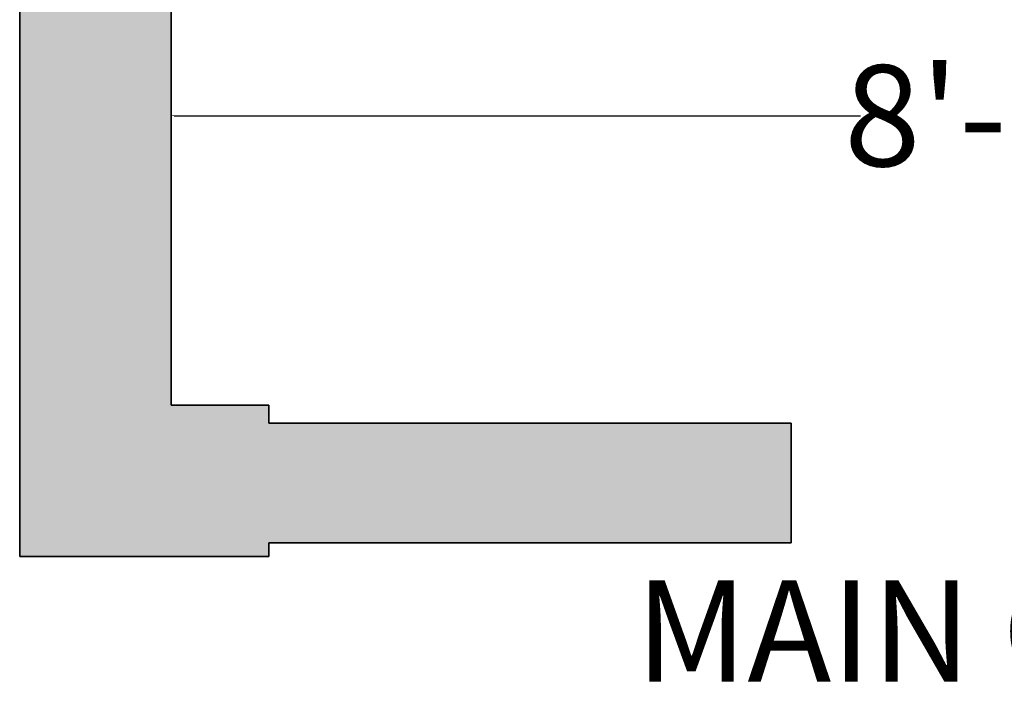
# Model space of a CAD drawing. Units: inches. Extents: x -5 to 482, y -460 to 66.
# Tile 1 of 31: x 33 to 91, y -429 to -390. Entities that reach past the tile are written whole.
import ezdxf

# ---------------------------------------------------------------- set-up
doc = ezdxf.new("R2010")
doc.units = ezdxf.units.IN
doc.header["$MEASUREMENT"] = 0
for name, color, linetype, lineweight in [('A-ANNO-DIMS', 2, 'Continuous', 18), ('A-ANNO-TEXT', 7, 'Continuous', 18), ('A-WALL', 7, 'Continuous', 35), ('A-WALL-PATT', 152, 'Continuous', 13)]:
    doc.layers.add(name, color=color, linetype=linetype, lineweight=lineweight)
doc.styles.get("Standard").update_dxf_attribs({"font": 'arial.ttf'})
doc.dimstyles.get("Standard").update_dxf_attribs({"dimtxt": 0.18, "dimasz": 0.18, "dimexe": 0.18, "dimexo": 0.0625, "dimgap": 0.09, "dimtad": 0, "dimtih": 1, "dimtoh": 1, "dimdec": 0, "dimzin": 0, "dimdsep": 46, "dimlunit": 3, "dimtxsty": 'Standard', "dimcen": 0.09, "dimadec": 0, "dimazin": 0, "dimtfac": 1, "dimtdec": 0, "dimtofl": 0, "dimtmove": 0, "dimatfit": 3, "dimfxl": 1, "dimtolj": 1, "dimtzin": 0, "dimarcsym": 0})

# ---------------------------------------------------------------- blocks, each defined once
blk = doc.blocks.new('*D22')
at = {"layer": 'A-ANNO-DIMS', "color": 0, "lineweight": -2, "transparency": 16777216}
for p, q in [((41.877, -395.603), (41.877, -395.485)), ((42.057, -395.665), (82.808, -395.665)), ((139.697, -395.665), (98.946, -395.665)), ((139.877, -395.603), (139.877, -395.485))]:
    blk.add_line(p, q, dxfattribs=at)
at = {"layer": 'A-ANNO-DIMS', "color": 0, "transparency": 16777216}
for points in [[(42.057, -395.635), (42.057, -395.695), (41.877, -395.665)], [(139.697, -395.635), (139.697, -395.695), (139.877, -395.665)]]:
    blk.add_solid(points, dxfattribs=at)
at = {"layer": 'Defpoints', "color": 0, "transparency": 16777216}
for p in [(41.877, -395.665), (139.877, -395.665), (139.877, -395.665)]:
    blk.add_point(p, dxfattribs=at)
at = {"layer": 'A-ANNO-DIMS', "color": 0, "transparency": 16777216, "insert": (90.877, -395.665), "char_height": 6, "attachment_point": 5}
blk.add_mtext('\\A1;8\'-2"', dxfattribs=at)

msp = doc.modelspace()

# ---------------------------------------------------------------- hatches: boundary and pattern name
at = {"layer": 'A-WALL-PATT'}
h = msp.add_hatch(color=256, dxfattribs=at)
h.dxf.hatch_style = 1
h.paths.add_polyline_path([(149.377, -412.849), (144.377, -412.849), (144.377, -283.849), (144.377, -279.349), (133.877, -279.349), (133.877, -283.849), (139.877, -283.849), (139.877, -412.849), (133.51, -412.849), (133.51, -413.916), (102.652, -413.916), (102.652, -421.02), (133.51, -421.02), (133.51, -421.849), (149.377, -421.849)])
h.paths.add_polyline_path([(226.054, -412.849), (218.877, -412.849), (218.877, -350.849), (262.877, -350.849), (262.877, -386.849), (267.377, -386.849), (267.377, -283.849), (270.377, -283.849), (270.377, -279.349), (244.877, -279.349), (244.877, -283.849), (262.877, -283.849), (262.877, -346.349), (218.877, -346.349), (218.877, -283.849), (220.877, -283.849), (220.877, -279.349), (214.377, -279.349), (214.377, -283.849), (214.377, -412.849), (209.377, -412.849), (209.377, -421.849), (226.054, -421.849)])
h.paths.add_polyline_path([(315.815, -412.849), (250.054, -412.849), (250.054, -421.849), (315.815, -421.849)])
h.paths.add_polyline_path([(430.377, -378.349), (421.377, -378.349), (421.377, -412.849), (375.815, -412.849), (375.815, -421.849), (430.377, -421.849)])
h.paths.add_polyline_path([(78.691, -413.916), (47.68, -413.916), (47.68, -412.849), (41.877, -412.849), (41.877, -283.849), (109.877, -283.849), (109.877, -279.349), (41.877, -279.349), (41.877, -241.849), (32.877, -241.849), (32.877, -421.849), (47.68, -421.849), (47.68, -421.02), (78.691, -421.02)])
h.paths.add_polyline_path([(41.877, -144.349), (154.377, -144.349), (154.377, -137.849), (149.877, -137.849), (149.877, -139.849), (41.877, -139.849), (41.877, -97.849), (32.877, -97.849), (32.877, -181.849), (41.877, -181.849)])
h.paths.add_polyline_path([(430.377, -241.849), (421.377, -241.849), (421.377, -279.349), (309.377, -279.349), (309.377, -170.349), (304.877, -170.349), (304.877, -279.349), (294.377, -279.349), (294.377, -283.849), (421.377, -283.849), (421.377, -318.349), (430.377, -318.349)])
h.paths.add_polyline_path([(430.377, -119.849), (421.377, -119.849), (421.377, -139.849), (419.377, -139.849), (419.377, -144.349), (421.377, -144.349), (421.377, -181.849), (430.377, -181.849)])
h.paths.add_polyline_path([(395.377, -139.849), (377.377, -139.849), (377.377, -75.849), (421.377, -75.849), (421.377, -95.849), (430.377, -95.849), (430.377, -45.599), (421.377, -45.599), (421.377, -71.349), (377.377, -71.349), (377.377, -22.849), (372.877, -22.849), (372.877, -139.849), (242.877, -139.849), (242.877, -137.849), (238.377, -137.849), (238.377, -144.349), (304.877, -144.349), (304.877, -146.349), (309.377, -146.349), (309.377, -144.349), (395.377, -144.349)])
h.paths.add_polyline_path([(65.877, 13.151), (32.877, 13.151), (32.877, -37.849), (41.877, -37.849), (41.877, 4.151), (65.877, 4.151)])
h.paths.add_polyline_path([(166.377, 13.151), (125.877, 13.151), (125.877, 4.151), (149.877, 4.151), (149.877, -113.849), (154.377, -113.849), (154.377, 4.151), (166.377, 4.151)])
h.paths.add_polyline_path([(277.877, 13.151), (226.377, 13.151), (226.377, 4.151), (238.377, 4.151), (238.377, -113.849), (242.877, -113.849), (242.877, 4.151), (277.877, 4.151)])
h.paths.add_polyline_path([(430.377, 13.151), (337.877, 13.151), (337.877, 4.151), (372.877, 4.151), (372.877, 1.151), (377.377, 1.151), (377.377, 4.151), (421.377, 4.151), (421.377, -21.599), (430.377, -21.599)])

# ---------------------------------------------------------------- linework, layer by layer
at = {"layer": 'A-WALL'}
for p, q in [((32.877, 13.151), (32.877, -421.849)), ((41.877, -283.849), (41.877, -412.849)), ((41.877, -412.849), (47.68, -412.849)), ((47.68, -412.849), (47.68, -413.916)), ((78.691, -413.916), (47.68, -413.916)), ((78.691, -413.916), (78.691, -421.02)), ((78.691, -421.02), (47.68, -421.02)), ((47.68, -421.02), (47.68, -421.849)), ((32.877, -421.849), (47.68, -421.849))]:
    msp.add_line(p, q, dxfattribs=at)

# ---------------------------------------------------------------- texts
at = {"layer": 'A-ANNO-TEXT', "insert": (69.447, -423.262), "char_height": 6, "attachment_point": 1}
msp.add_mtext('MAIN GATE', dxfattribs=at)

# ---------------------------------------------------------------- dimensions: what is measured, and where the dimension line sits
at = {"layer": 'A-ANNO-DIMS'}
dim = msp.add_linear_dim(base=(139.877, -395.665), p1=(41.877, -395.665), p2=(139.877, -395.665), dimstyle='Standard', override={"dimtxt": 6, "dimclrd": 0, "dimclre": 0, "dimclrt": 0}, dxfattribs=at)
dim.commit()
dim.dimension.update_dxf_attribs({"geometry": '*D22', "text_midpoint": (90.877, -395.665)})

doc.saveas('drawing.dxf')
